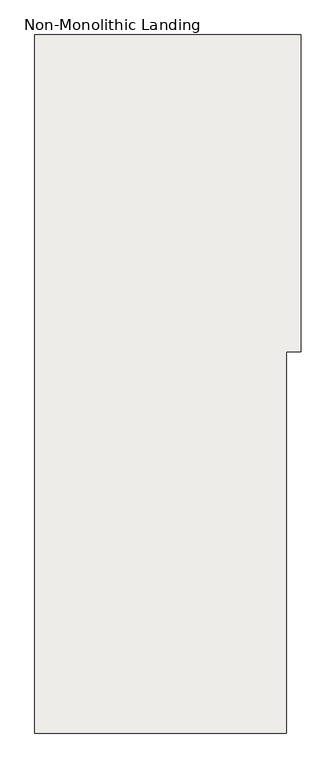
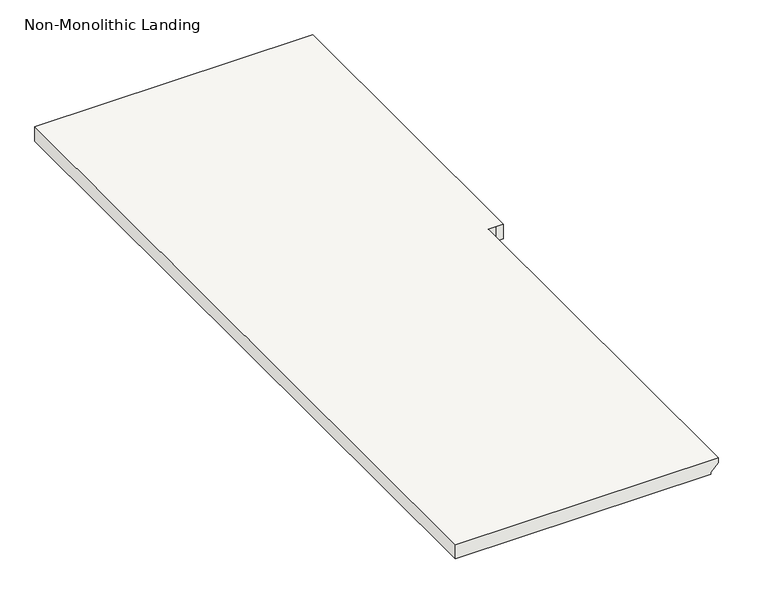
"""IFC4 building model written with IfcOpenShell, lengths in millimetres: slab geometry, Non-Monolithic Landing."""

from ifc_helpers import new_model, si_unit, origin, place, context, project, spatial, faceted_brep, source, transform, mapped, element, save


def non_monolithic_landing_c221236f(model_context):
    return source(origin(), model_context, "Body", "Brep", [
        faceted_brep([(-10221.4683044, -3838.3891189, 1581.15), (-10246.8683044, -3838.3891189, 1555.75), (-10246.8683044, -2706.1923176, 1555.75), (-10221.4683044, -2706.1923176, 1581.15), (-10221.4683044, -2492.1891189, 1600.2), (-10196.0683044, -2492.1891189, 1600.2), (-10170.6683044, -2492.1891189, 1600.2), (-10170.6683044, -1374.5891189, 1600.2), (-10196.0683044, -1374.5891189, 1600.2), (-11110.4683044, -1374.5891189, 1600.2), (-11110.4683044, -3838.3891189, 1600.2), (-10221.4683044, -3838.3891189, 1600.2), (-10246.8683044, -2706.1923176, 1549.4), (-10246.8683044, -3838.3891189, 1549.4), (-11110.4683044, -3838.3891189, 1549.4), (-11110.4683044, -1374.5891189, 1549.4), (-10196.0683044, -1374.5891189, 1549.4), (-10170.6683044, -1374.5891189, 1549.4), (-10170.6683044, -2492.1891189, 1549.4), (-10196.0683044, -2492.1891189, 1549.4), (-10221.4683044, -2492.1891189, 1549.4), (-10221.4683044, -2706.1923176, 1549.4)], [[[0, 1, 2, 3]], [[4, 5, 6, 7, 8, 9, 10, 11]], [[12, 13, 14, 15, 16, 17, 18, 19, 20, 21]], [[13, 12, 2, 1]], [[12, 21, 3, 2]], [[4, 11, 0, 3, 21, 20]], [[9, 8, 16, 15]], [[10, 9, 15, 14]], [[11, 10, 14, 13, 1, 0]], [[5, 4, 20, 19]], [[6, 5, 19, 18]], [[7, 6, 18, 17]], [[8, 7, 17, 16]]]),
    ])


if __name__ == "__main__":
    model = new_model("IFC4")
    model_context = context("Model", 3, world=origin())
    ifc_project = project(units=[si_unit("LENGTHUNIT", "METRE", prefix="MILLI")], contexts=[model_context])
    site = spatial("IfcSite", under=ifc_project)
    building = spatial("IfcBuilding", under=site)
    placement = place(None, origin())
    non_monolithic_landing_shape = non_monolithic_landing_c221236f(model_context)
    element("IfcSlab", 1, ObjectType="Non-Monolithic Landing", at=placement, inside=building, context=model_context, shape_type="MappedRepresentation", body=[
        mapped(non_monolithic_landing_shape, transform((0.0, 0.0, 0.0), x_axis=(1.0, 0.0, 0.0), y_axis=(0.0, 1.0, 0.0), z_axis=(0.0, 0.0, 1.0))),
    ])
    save(model, "model.ifc")
